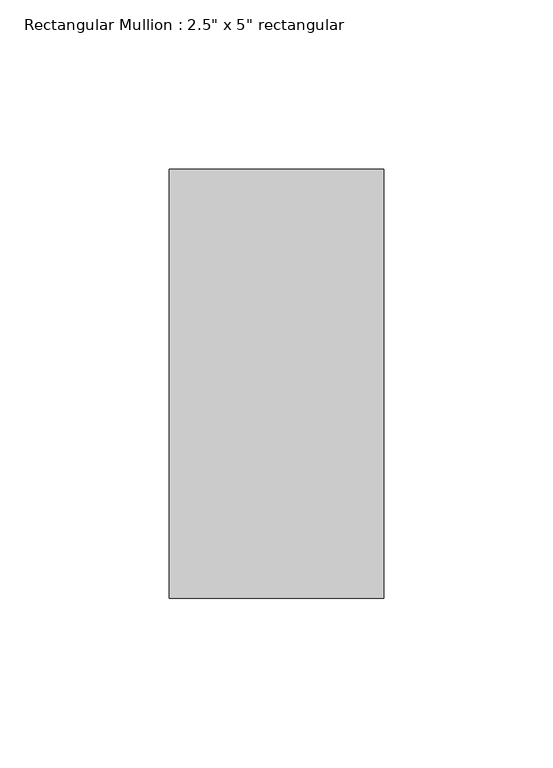
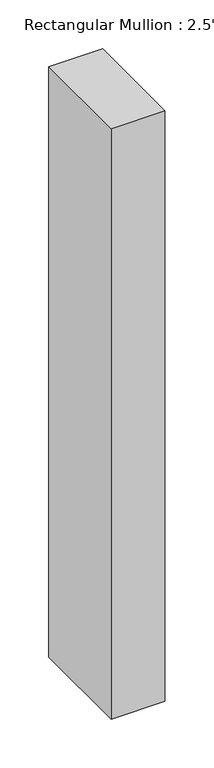
"""IFC4 building model written with IfcOpenShell, lengths in millimetres: member geometry."""

from ifc_helpers import new_model, si_unit, frame, origin, place, context, project, spatial, polyline, outline, extrude, source, transform, mapped, element, save


def member_d7af48b5(model_context):
    return source(origin(), model_context, "Body", "SweptSolid", [
        extrude(outline(polyline([(0.0, 63.5), (0.0, -63.5), (-63.5, -63.5), (-63.5, 63.5), (0.0, 63.5)])), frame((0.0, 0.0, -736.6), z_axis=(0.0, 0.0, 1.0), x_axis=(1.0, 0.0, 0.0)), (0.0, 0.0, 1.0), 736.6),
    ])


if __name__ == "__main__":
    model = new_model("IFC4")
    model_context = context("Model", 3, world=origin())
    ifc_project = project(units=[si_unit("LENGTHUNIT", "METRE", prefix="MILLI")], contexts=[model_context])
    site = spatial("IfcSite", under=ifc_project)
    building = spatial("IfcBuilding", under=site)
    placement = place(None, origin())
    member_shape = member_d7af48b5(model_context)
    element("IfcMember", 1, ObjectType="Rectangular Mullion : 2.5\" x 5\" rectangular", at=placement, inside=building, context=model_context, shape_type="MappedRepresentation", body=[
        mapped(member_shape, transform((0.0, 0.0, 0.0), x_axis=(1.0, 0.0, 0.0), y_axis=(0.0, 1.0, 0.0), z_axis=(0.0, 0.0, 1.0))),
    ])
    save(model, "model.ifc")

# Revit data of these elements
# Type "Rectangular Mullion : 2.5\" x 5\" rectangular"
#   built-in parameter 1007304 = 0.416667 (stored number, unit not read)
#   built-in parameter 1007301 = 0.104167 (stored number, unit not read)
#   built-in parameter 1007300 = 0.104167 (stored number, unit not read)
# Element 1 (IfcMember, "Rectangular Mullion : 2.5\" x 5\" rectangular")
#   Materials on its faces: "Aluminum"
# Materials
#   "Aluminum": class "Metal", colour RGB 247 247 247, transparency 0, Description = "Aluminum 6061", Cost = 0
